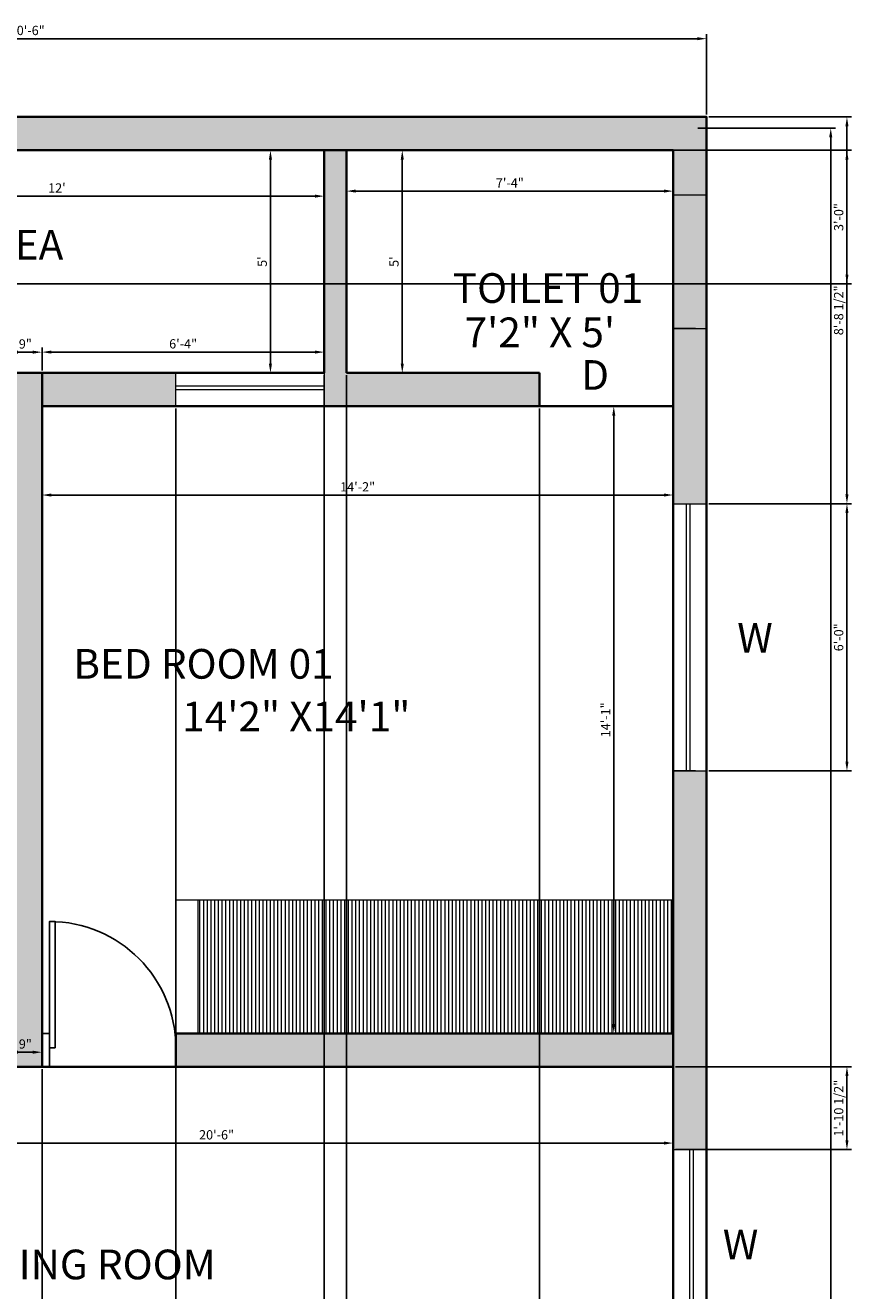
# Model space of a CAD drawing. Units: inches. Extents: x 844 to 1293, y 1224 to 2014.
# Tile 4 of 4: x 1070 to 1293, y 1673 to 2014. Entities that reach past the tile are written whole.
import ezdxf

# ---------------------------------------------------------------- set-up
doc = ezdxf.new("R2010")
doc.units = ezdxf.units.IN
for name, color, linetype, lineweight in [('A-ANNO-DIMS', 2, 'Continuous', 18), ('A-ANNO-TEXT', 3, 'Continuous', 18), ('A-AREA-IDEN', 7, 'Continuous', 25), ('A-DOOR', 3, 'Continuous', 25), ('A-FLOR-PATT', 8, 'Continuous', 13), ('A-GLAZ', 4, 'Continuous', 18), ('A-WALL', 7, 'Continuous', 35), ('A-WALL-PATT', 252, 'Continuous', 13)]:
    doc.layers.add(name, color=color, linetype=linetype, lineweight=lineweight)
doc.styles.get("Standard").update_dxf_attribs({"font": 'arial.ttf'})
doc.dimstyles.new('Copy of ISO-25', dxfattribs={"dimtxt": 2.5, "dimasz": 2.5, "dimexe": 1.25, "dimexo": 0.625, "dimtad": 1, "dimlunit": 4, "dimtxsty": 'Standard', "dimcen": 2.5, "dimadec": 0, "dimazin": 0, "dimtfac": 1, "dimtmove": 0, "dimatfit": 3, "dimfxl": 1, "dimarcsym": 0})

# ---------------------------------------------------------------- blocks, each defined once
blk = doc.blocks.new('*U3')
for p, q in [((0, 0), (0, -6)), ((40, 0), (40, -6))]:
    blk.add_line(p, q)
blk.add_lwpolyline([(0, 0), (0, 40), (1.75, 40), (1.75, 0)], close=True)
blk.add_arc((0, 0), 40, 0, 90)
blk = doc.blocks.new('*D5')
at = {"layer": 'A-ANNO-DIMS', "color": 0, "lineweight": -2, "transparency": 16777216}
for p, q in [((1074.46, 1910.42), (1074.46, 1885.88)), ((1244.46, 1910.42), (1244.46, 1885.88)), ((1076.96, 1887.13), (1241.96, 1887.13))]:
    blk.add_line(p, q, dxfattribs=at)
at = {"layer": 'A-ANNO-DIMS', "color": 0, "transparency": 16777216}
for points in [[(1076.96, 1887.54), (1076.96, 1886.71), (1074.46, 1887.13)], [(1241.96, 1887.54), (1241.96, 1886.71), (1244.46, 1887.13)]]:
    blk.add_solid(points, dxfattribs=at)
at = {"layer": 'Defpoints', "color": 0, "transparency": 16777216}
for p in [(1074.46, 1911.04), (1244.46, 1911.04), (1244.46, 1887.13)]:
    blk.add_point(p, dxfattribs=at)
at = {"layer": 'A-ANNO-DIMS', "color": 0, "transparency": 16777216, "insert": (1159.46, 1889.01), "char_height": 2.5, "attachment_point": 5}
blk.add_mtext('14\'-2"', dxfattribs=at)
blk = doc.blocks.new('*D6')
at = {"layer": 'A-ANNO-DIMS', "color": 0, "lineweight": -2, "transparency": 16777216}
for p, q in [((1243.84, 1911.04), (1227.21, 1911.04)), ((1228.46, 1908.54), (1228.46, 1744.54)), ((1243.84, 1742.04), (1227.21, 1742.04))]:
    blk.add_line(p, q, dxfattribs=at)
at = {"layer": 'A-ANNO-DIMS', "color": 0, "transparency": 16777216}
for points in [[(1228.05, 1908.54), (1228.88, 1908.54), (1228.46, 1911.04)], [(1228.05, 1744.54), (1228.88, 1744.54), (1228.46, 1742.04)]]:
    blk.add_solid(points, dxfattribs=at)
at = {"layer": 'Defpoints', "color": 0, "transparency": 16777216}
for p in [(1244.46, 1911.04), (1228.46, 1742.04), (1244.46, 1742.04)]:
    blk.add_point(p, dxfattribs=at)
at = {"layer": 'A-ANNO-DIMS', "color": 0, "transparency": 16777216, "insert": (1226.58, 1826.54), "char_height": 2.5, "attachment_point": 5, "rotation": 90}
blk.add_mtext('14\'-1"', dxfattribs=at)
blk = doc.blocks.new('*D11')
at = {"layer": 'A-ANNO-DIMS', "color": 0, "lineweight": -2, "transparency": 16777216}
for p, q in [((1006.46, 1979.42), (1006.46, 1966.44)), ((1150.46, 1979.42), (1150.46, 1966.44)), ((1008.96, 1967.69), (1147.96, 1967.69))]:
    blk.add_line(p, q, dxfattribs=at)
at = {"layer": 'A-ANNO-DIMS', "color": 0, "transparency": 16777216}
for points in [[(1008.96, 1968.11), (1008.96, 1967.27), (1006.46, 1967.69)], [(1147.96, 1968.11), (1147.96, 1967.27), (1150.46, 1967.69)]]:
    blk.add_solid(points, dxfattribs=at)
at = {"layer": 'Defpoints', "color": 0, "transparency": 16777216}
for p in [(1006.46, 1980.04), (1150.46, 1980.04), (1150.46, 1967.69)]:
    blk.add_point(p, dxfattribs=at)
at = {"layer": 'A-ANNO-DIMS', "color": 0, "transparency": 16777216, "insert": (1078.46, 1969.57), "char_height": 2.5, "attachment_point": 5}
blk.add_mtext("12'", dxfattribs=at)
blk = doc.blocks.new('*D12')
at = {"layer": 'A-ANNO-DIMS', "color": 0, "lineweight": -2, "transparency": 16777216}
for p, q in [((1149.84, 1980.04), (1134.73, 1980.04)), ((1135.98, 1922.54), (1135.98, 1977.54)), ((1149.84, 1920.04), (1134.73, 1920.04))]:
    blk.add_line(p, q, dxfattribs=at)
at = {"layer": 'A-ANNO-DIMS', "color": 0, "transparency": 16777216}
for points in [[(1135.56, 1977.54), (1136.39, 1977.54), (1135.98, 1980.04)], [(1135.56, 1922.54), (1136.39, 1922.54), (1135.98, 1920.04)]]:
    blk.add_solid(points, dxfattribs=at)
at = {"layer": 'Defpoints', "color": 0, "transparency": 16777216}
for p in [(1135.98, 1980.04), (1150.46, 1980.04), (1150.46, 1920.04)]:
    blk.add_point(p, dxfattribs=at)
at = {"layer": 'A-ANNO-DIMS', "color": 0, "transparency": 16777216, "insert": (1134.08, 1950.04), "char_height": 2.5, "attachment_point": 5, "rotation": 90}
blk.add_mtext("5'", dxfattribs=at)
blk = doc.blocks.new('*D13')
at = {"layer": 'A-ANNO-DIMS', "color": 0, "lineweight": -2, "transparency": 16777216}
for p, q in [((1156.46, 1979.42), (1156.46, 1967.79)), ((1244.46, 1979.42), (1244.46, 1967.79)), ((1158.96, 1969.04), (1241.96, 1969.04))]:
    blk.add_line(p, q, dxfattribs=at)
at = {"layer": 'A-ANNO-DIMS', "color": 0, "transparency": 16777216}
for points in [[(1158.96, 1969.46), (1158.96, 1968.63), (1156.46, 1969.04)], [(1241.96, 1969.46), (1241.96, 1968.63), (1244.46, 1969.04)]]:
    blk.add_solid(points, dxfattribs=at)
at = {"layer": 'Defpoints', "color": 0, "transparency": 16777216}
for p in [(1156.46, 1980.04), (1244.46, 1980.04), (1244.46, 1969.04)]:
    blk.add_point(p, dxfattribs=at)
at = {"layer": 'A-ANNO-DIMS', "color": 0, "transparency": 16777216, "insert": (1200.46, 1970.92), "char_height": 2.5, "attachment_point": 5}
blk.add_mtext('7\'-4"', dxfattribs=at)
blk = doc.blocks.new('*D14')
at = {"layer": 'A-ANNO-DIMS', "color": 0, "lineweight": -2, "transparency": 16777216}
for p, q in [((1157.09, 1980.04), (1172.74, 1980.04)), ((1171.49, 1977.54), (1171.49, 1922.54)), ((1157.09, 1920.04), (1172.74, 1920.04))]:
    blk.add_line(p, q, dxfattribs=at)
at = {"layer": 'A-ANNO-DIMS', "color": 0, "transparency": 16777216}
for points in [[(1171.07, 1977.54), (1171.91, 1977.54), (1171.49, 1980.04)], [(1171.07, 1922.54), (1171.91, 1922.54), (1171.49, 1920.04)]]:
    blk.add_solid(points, dxfattribs=at)
at = {"layer": 'Defpoints', "color": 0, "transparency": 16777216}
for p in [(1156.46, 1980.04), (1156.46, 1920.04), (1171.49, 1920.04)]:
    blk.add_point(p, dxfattribs=at)
at = {"layer": 'A-ANNO-DIMS', "color": 0, "transparency": 16777216, "insert": (1169.59, 1950.04), "char_height": 2.5, "attachment_point": 5, "rotation": 90}
blk.add_mtext("5'", dxfattribs=at)
blk = doc.blocks.new('*D18')
at = {"layer": 'A-ANNO-DIMS', "color": 0, "lineweight": -2, "transparency": 16777216}
for p, q in [((998.46, 1732.42), (998.46, 1711.23)), ((1244.46, 1732.42), (1244.46, 1711.23)), ((1000.96, 1712.48), (1241.96, 1712.48))]:
    blk.add_line(p, q, dxfattribs=at)
at = {"layer": 'A-ANNO-DIMS', "color": 0, "transparency": 16777216}
for points in [[(1000.96, 1712.89), (1000.96, 1712.06), (998.46, 1712.48)], [(1241.96, 1712.89), (1241.96, 1712.06), (1244.46, 1712.48)]]:
    blk.add_solid(points, dxfattribs=at)
at = {"layer": 'Defpoints', "color": 0, "transparency": 16777216}
for p in [(998.46, 1733.04), (1244.46, 1733.04), (1244.46, 1712.48)]:
    blk.add_point(p, dxfattribs=at)
at = {"layer": 'A-ANNO-DIMS', "color": 0, "transparency": 16777216, "insert": (1121.46, 1714.38), "char_height": 2.5, "attachment_point": 5}
blk.add_mtext('20\'-6"', dxfattribs=at)
blk = doc.blocks.new('*D20')
at = {"layer": 'A-ANNO-DIMS', "color": 0, "lineweight": -2, "transparency": 16777216}
for p, q in [((1251.09, 1986.04), (1288.15, 1986.04)), ((1286.9, 1983.54), (1286.9, 1268.54)), ((1251.09, 1266.04), (1288.15, 1266.04))]:
    blk.add_line(p, q, dxfattribs=at)
at = {"layer": 'A-ANNO-DIMS', "color": 0, "transparency": 16777216}
for points in [[(1286.48, 1983.54), (1287.31, 1983.54), (1286.9, 1986.04)], [(1286.48, 1268.54), (1287.31, 1268.54), (1286.9, 1266.04)]]:
    blk.add_solid(points, dxfattribs=at)
at = {"layer": 'Defpoints', "color": 0, "transparency": 16777216}
for p in [(1250.46, 1986.04), (1250.46, 1266.04), (1286.9, 1266.04)]:
    blk.add_point(p, dxfattribs=at)
at = {"layer": 'A-ANNO-DIMS', "color": 0, "transparency": 16777216, "insert": (1285, 1626.04), "char_height": 2.5, "attachment_point": 5, "rotation": 90}
blk.add_mtext("60'", dxfattribs=at)
blk = doc.blocks.new('*D27')
at = {"layer": 'A-ANNO-DIMS', "color": 0, "lineweight": -2, "transparency": 16777216}
for p, q in [((1074.46, 1920.67), (1074.46, 1926.9)), ((1150.46, 1920.67), (1150.46, 1926.9)), ((1076.96, 1925.65), (1147.96, 1925.65))]:
    blk.add_line(p, q, dxfattribs=at)
at = {"layer": 'A-ANNO-DIMS', "color": 0, "transparency": 16777216}
for points in [[(1076.96, 1926.07), (1076.96, 1925.24), (1074.46, 1925.65)], [(1147.96, 1926.07), (1147.96, 1925.24), (1150.46, 1925.65)]]:
    blk.add_solid(points, dxfattribs=at)
at = {"layer": 'Defpoints', "color": 0, "transparency": 16777216}
for p in [(1150.46, 1925.65), (1074.46, 1920.04), (1150.46, 1920.04)]:
    blk.add_point(p, dxfattribs=at)
at = {"layer": 'A-ANNO-DIMS', "color": 0, "transparency": 16777216, "insert": (1112.46, 1927.56), "char_height": 2.5, "attachment_point": 5}
blk.add_mtext('6\'-4"', dxfattribs=at)
blk = doc.blocks.new('*D30')
at = {"layer": 'A-ANNO-DIMS', "color": 0, "lineweight": -2, "transparency": 16777216}
for p, q in [((887.46, 1989.67), (887.46, 2011.37)), ((889.96, 2010.12), (1250.96, 2010.12)), ((1253.46, 1989.67), (1253.46, 2011.37))]:
    blk.add_line(p, q, dxfattribs=at)
at = {"layer": 'A-ANNO-DIMS', "color": 0, "transparency": 16777216}
for points in [[(889.96, 2010.54), (889.96, 2009.71), (887.46, 2010.12)], [(1250.96, 2010.54), (1250.96, 2009.71), (1253.46, 2010.12)]]:
    blk.add_solid(points, dxfattribs=at)
at = {"layer": 'Defpoints', "color": 0, "transparency": 16777216}
for p in [(1253.46, 2010.12), (887.46, 1989.04), (1253.46, 1989.04)]:
    blk.add_point(p, dxfattribs=at)
at = {"layer": 'A-ANNO-DIMS', "color": 0, "transparency": 16777216, "insert": (1070.46, 2012.02), "char_height": 2.5, "attachment_point": 5}
blk.add_mtext('30\'-6"', dxfattribs=at)
blk = doc.blocks.new('*D34')
at = {"layer": 'A-ANNO-DIMS', "color": 0, "lineweight": -2, "transparency": 16777216}
for p, q in [((1065.46, 1920.67), (1065.46, 1926.88)), ((1074.46, 1920.67), (1074.46, 1926.88)), ((1067.96, 1925.63), (1071.96, 1925.63))]:
    blk.add_line(p, q, dxfattribs=at)
at = {"layer": 'A-ANNO-DIMS', "color": 0, "transparency": 16777216}
for points in [[(1067.96, 1926.05), (1067.96, 1925.22), (1065.46, 1925.63)], [(1071.96, 1926.05), (1071.96, 1925.22), (1074.46, 1925.63)]]:
    blk.add_solid(points, dxfattribs=at)
at = {"layer": 'Defpoints', "color": 0, "transparency": 16777216}
for p in [(1074.46, 1925.63), (1065.46, 1920.04), (1074.46, 1920.04)]:
    blk.add_point(p, dxfattribs=at)
at = {"layer": 'A-ANNO-DIMS', "color": 0, "transparency": 16777216, "insert": (1069.96, 1927.53), "char_height": 2.5, "attachment_point": 5}
blk.add_mtext('9"', dxfattribs=at)
blk = doc.blocks.new('*D36')
at = {"layer": 'A-ANNO-DIMS', "color": 0, "lineweight": -2, "transparency": 16777216}
for p, q in [((1065.46, 1733.67), (1065.46, 1738.21)), ((1067.96, 1736.96), (1071.96, 1736.96)), ((1074.46, 1733.67), (1074.46, 1738.21))]:
    blk.add_line(p, q, dxfattribs=at)
at = {"layer": 'A-ANNO-DIMS', "color": 0, "transparency": 16777216}
for points in [[(1067.96, 1737.38), (1067.96, 1736.54), (1065.46, 1736.96)], [(1071.96, 1737.38), (1071.96, 1736.54), (1074.46, 1736.96)]]:
    blk.add_solid(points, dxfattribs=at)
at = {"layer": 'Defpoints', "color": 0, "transparency": 16777216}
for p in [(1074.46, 1736.96), (1065.46, 1733.04), (1074.46, 1733.04)]:
    blk.add_point(p, dxfattribs=at)
at = {"layer": 'A-ANNO-DIMS', "color": 0, "transparency": 16777216, "insert": (1069.96, 1738.86), "char_height": 2.5, "attachment_point": 5}
blk.add_mtext('9"', dxfattribs=at)
blk = doc.blocks.new('WIN-GLAZ-60IN')
for p, q in [((0, 60), (0, 0)), ((1, 60), (1, 0))]:
    blk.add_line(p, q)
blk = doc.blocks.new('*D55')
at = {"layer": 'A-ANNO-DIMS', "color": 0, "lineweight": -2, "transparency": 16777216}
for p, q in [((1254.09, 1989.04), (1292.51, 1989.04)), ((1291.26, 1887.28), (1291.26, 1986.54)), ((1254.09, 1884.78), (1292.51, 1884.78))]:
    blk.add_line(p, q, dxfattribs=at)
at = {"layer": 'A-ANNO-DIMS', "color": 0, "transparency": 16777216}
for points in [[(1290.85, 1986.54), (1291.68, 1986.54), (1291.26, 1989.04)], [(1290.85, 1887.28), (1291.68, 1887.28), (1291.26, 1884.78)]]:
    blk.add_solid(points, dxfattribs=at)
at = {"layer": 'Defpoints', "color": 0, "transparency": 16777216}
for p in [(1253.46, 1989.04), (1291.26, 1989.04), (1253.46, 1884.78)]:
    blk.add_point(p, dxfattribs=at)
at = {"layer": 'A-ANNO-DIMS', "color": 0, "transparency": 16777216, "insert": (1289.35, 1936.91), "char_height": 2.5, "attachment_point": 5, "rotation": 90}
blk.add_mtext('8\'-8 1/2"', dxfattribs=at)
blk = doc.blocks.new('*D56')
at = {"layer": 'A-ANNO-DIMS', "color": 0, "lineweight": -2, "transparency": 16777216}
for p, q in [((1254.09, 1884.78), (1292.51, 1884.78)), ((1291.26, 1815.28), (1291.26, 1882.28)), ((1254.09, 1812.78), (1292.51, 1812.78))]:
    blk.add_line(p, q, dxfattribs=at)
at = {"layer": 'A-ANNO-DIMS', "color": 0, "transparency": 16777216}
for points in [[(1290.85, 1882.28), (1291.68, 1882.28), (1291.26, 1884.78)], [(1290.85, 1815.28), (1291.68, 1815.28), (1291.26, 1812.78)]]:
    blk.add_solid(points, dxfattribs=at)
at = {"layer": 'Defpoints', "color": 0, "transparency": 16777216}
for p in [(1253.46, 1884.78), (1291.26, 1884.78), (1253.46, 1812.78)]:
    blk.add_point(p, dxfattribs=at)
at = {"layer": 'A-ANNO-DIMS', "color": 0, "transparency": 16777216, "insert": (1289.36, 1848.78), "char_height": 2.5, "attachment_point": 5, "rotation": 90}
blk.add_mtext('6\'-0"', dxfattribs=at)
blk = doc.blocks.new('*D58')
at = {"layer": 'A-ANNO-DIMS', "color": 0, "lineweight": -2, "transparency": 16777216}
for p, q in [((1245.09, 1733.04), (1292.51, 1733.04)), ((1291.26, 1713.23), (1291.26, 1730.54)), ((1245.09, 1710.73), (1292.51, 1710.73))]:
    blk.add_line(p, q, dxfattribs=at)
at = {"layer": 'A-ANNO-DIMS', "color": 0, "transparency": 16777216}
for points in [[(1290.85, 1730.54), (1291.68, 1730.54), (1291.26, 1733.04)], [(1290.85, 1713.23), (1291.68, 1713.23), (1291.26, 1710.73)]]:
    blk.add_solid(points, dxfattribs=at)
at = {"layer": 'Defpoints', "color": 0, "transparency": 16777216}
for p in [(1244.46, 1733.04), (1291.26, 1733.04), (1244.46, 1710.73)]:
    blk.add_point(p, dxfattribs=at)
at = {"layer": 'A-ANNO-DIMS', "color": 0, "transparency": 16777216, "insert": (1289.35, 1721.88), "char_height": 2.5, "attachment_point": 5, "rotation": 90}
blk.add_mtext('1\'-10 1/2"', dxfattribs=at)
blk = doc.blocks.new('*D63')
at = {"layer": 'A-ANNO-DIMS', "color": 0, "lineweight": -2, "transparency": 16777216}
for p, q in [((1110.46, 1910.42), (1110.46, 1223.99)), ((1150.46, 1910.42), (1150.46, 1223.99)), ((1112.96, 1225.24), (1147.96, 1225.24))]:
    blk.add_line(p, q, dxfattribs=at)
at = {"layer": 'A-ANNO-DIMS', "color": 0, "transparency": 16777216}
for points in [[(1112.96, 1225.66), (1112.96, 1224.82), (1110.46, 1225.24)], [(1147.96, 1225.66), (1147.96, 1224.82), (1150.46, 1225.24)]]:
    blk.add_solid(points, dxfattribs=at)
at = {"layer": 'Defpoints', "color": 0, "transparency": 16777216}
for p in [(1110.46, 1911.04), (1150.46, 1911.04), (1150.46, 1225.24)]:
    blk.add_point(p, dxfattribs=at)
at = {"layer": 'A-ANNO-DIMS', "color": 0, "transparency": 16777216, "insert": (1130.46, 1227.14), "char_height": 2.5, "attachment_point": 5}
blk.add_mtext('3\'-4"', dxfattribs=at)
blk = doc.blocks.new('*D64')
at = {"layer": 'A-ANNO-DIMS', "color": 0, "lineweight": -2, "transparency": 16777216}
for p, q in [((1208.46, 1910.42), (1208.46, 1223.99)), ((1244.46, 1910.42), (1244.46, 1223.99)), ((1210.96, 1225.24), (1241.96, 1225.24))]:
    blk.add_line(p, q, dxfattribs=at)
at = {"layer": 'A-ANNO-DIMS', "color": 0, "transparency": 16777216}
for points in [[(1210.96, 1225.66), (1210.96, 1224.82), (1208.46, 1225.24)], [(1241.96, 1225.66), (1241.96, 1224.82), (1244.46, 1225.24)]]:
    blk.add_solid(points, dxfattribs=at)
at = {"layer": 'Defpoints', "color": 0, "transparency": 16777216}
for p in [(1208.46, 1911.04), (1244.46, 1911.04), (1244.46, 1225.24)]:
    blk.add_point(p, dxfattribs=at)
at = {"layer": 'A-ANNO-DIMS', "color": 0, "transparency": 16777216, "insert": (1226.46, 1227.14), "char_height": 2.5, "attachment_point": 5}
blk.add_mtext('3\'-0"', dxfattribs=at)
blk = doc.blocks.new('*D65')
at = {"layer": 'A-ANNO-DIMS', "color": 0, "lineweight": -2, "transparency": 16777216}
for p, q in [((1007.09, 1980.04), (1292.51, 1980.04)), ((1291.26, 1946.54), (1291.26, 1977.54)), ((1001.09, 1944.04), (1292.51, 1944.04))]:
    blk.add_line(p, q, dxfattribs=at)
at = {"layer": 'A-ANNO-DIMS', "color": 0, "transparency": 16777216}
for points in [[(1290.85, 1977.54), (1291.68, 1977.54), (1291.26, 1980.04)], [(1290.85, 1946.54), (1291.68, 1946.54), (1291.26, 1944.04)]]:
    blk.add_solid(points, dxfattribs=at)
at = {"layer": 'Defpoints', "color": 0, "transparency": 16777216}
for p in [(1006.46, 1980.04), (1291.26, 1980.04), (1000.46, 1944.04)]:
    blk.add_point(p, dxfattribs=at)
at = {"layer": 'A-ANNO-DIMS', "color": 0, "transparency": 16777216, "insert": (1289.36, 1962.04), "char_height": 2.5, "attachment_point": 5, "rotation": 90}
blk.add_mtext('3\'-0"', dxfattribs=at)
blk = doc.blocks.new('*D67')
at = {"layer": 'A-ANNO-DIMS', "color": 0, "lineweight": -2, "transparency": 16777216}
for p, q in [((1074.46, 1732.42), (1074.46, 1223.99)), ((1110.46, 1732.42), (1110.46, 1223.99)), ((1076.96, 1225.24), (1107.96, 1225.24))]:
    blk.add_line(p, q, dxfattribs=at)
at = {"layer": 'A-ANNO-DIMS', "color": 0, "transparency": 16777216}
for points in [[(1076.96, 1225.66), (1076.96, 1224.82), (1074.46, 1225.24)], [(1107.96, 1225.66), (1107.96, 1224.82), (1110.46, 1225.24)]]:
    blk.add_solid(points, dxfattribs=at)
at = {"layer": 'Defpoints', "color": 0, "transparency": 16777216}
for p in [(1074.46, 1733.04), (1110.46, 1733.04), (1110.46, 1225.24)]:
    blk.add_point(p, dxfattribs=at)
at = {"layer": 'A-ANNO-DIMS', "color": 0, "transparency": 16777216, "insert": (1092.46, 1227.14), "char_height": 2.5, "attachment_point": 5}
blk.add_mtext('3\'-0"', dxfattribs=at)
blk = doc.blocks.new('*D73')
at = {"layer": 'A-ANNO-DIMS', "color": 0, "lineweight": -2, "transparency": 16777216}
for p, q in [((1150.46, 1919.42), (1150.46, 1223.99)), ((1156.46, 1919.42), (1156.46, 1223.99)), ((1147.96, 1225.24), (1145.46, 1225.24)), ((1150.46, 1225.24), (1156.46, 1225.24)), ((1158.96, 1225.24), (1169.36, 1225.24))]:
    blk.add_line(p, q, dxfattribs=at)
at = {"layer": 'A-ANNO-DIMS', "color": 0, "transparency": 16777216}
for points in [[(1147.96, 1225.66), (1147.96, 1224.82), (1150.46, 1225.24)], [(1158.96, 1225.66), (1158.96, 1224.82), (1156.46, 1225.24)]]:
    blk.add_solid(points, dxfattribs=at)
at = {"layer": 'Defpoints', "color": 0, "transparency": 16777216}
for p in [(1150.46, 1920.04), (1156.46, 1920.04), (1156.46, 1225.24)]:
    blk.add_point(p, dxfattribs=at)
at = {"layer": 'A-ANNO-DIMS', "color": 0, "transparency": 16777216, "insert": (1165.41, 1227.14), "char_height": 2.5, "attachment_point": 5}
blk.add_mtext('0\'-6"', dxfattribs=at)

msp = doc.modelspace()

# ---------------------------------------------------------------- hatches: boundary and pattern name
at = {"layer": 'A-FLOR-PATT'}
h = msp.add_hatch(dxfattribs=at)
h.set_pattern_fill('ANSI31', color=256, scale=0.3149606, angle=45, style=0)
h.paths.add_polyline_path([(1116.465, 1742.042), (1244.465, 1742.042), (1244.465, 1778.042), (1116.465, 1778.042)])
at = {"layer": 'A-WALL-PATT'}
h = msp.add_hatch(color=256, dxfattribs=at)
h.dxf.hatch_style = 1
h.paths.add_polyline_path([(1253.465, 1989.042), (887.465, 1989.042), (887.465, 1920.042), (887.465, 1911.042), (887.465, 1871.621), (896.465, 1871.621), (896.465, 1911.042), (896.465, 1920.042), (896.465, 1980.042), (1000.465, 1980.042), (1244.465, 1980.042), (1244.465, 1968.042), (1253.465, 1968.042)])
h.paths.add_polyline_path([(1006.465, 1944.042), (1000.465, 1944.042), (1000.465, 1920.042), (896.465, 1920.042), (896.465, 1911.042), (1006.465, 1911.042), (1006.465, 1920.042)], flags=17)
h.paths.add_polyline_path([(1253.465, 1968.042), (1244.465, 1968.042), (1244.465, 1932.042), (1253.465, 1932.042)], flags=17)
h.paths.add_polyline_path([(1253.465, 1920.042), (1253.465, 1932.042), (1244.465, 1932.042), (1244.465, 1920.042), (1244.465, 1911.042), (1244.465, 1884.775), (1253.465, 1884.775), (1253.465, 1911.042)], flags=17)
h.paths.add_polyline_path([(1208.465, 1920.042), (1156.465, 1920.042), (1156.465, 1980.042), (1150.465, 1980.042), (1150.465, 1920.042), (1150.465, 1911.042), (1208.465, 1911.042)], flags=17)
h.paths.add_polyline_path([(1110.465, 1920.042), (1074.465, 1920.042), (1074.465, 1911.042), (1110.465, 1911.042)], flags=17)
h.paths.add_polyline_path([(896.465, 1811.621), (887.465, 1811.621), (887.465, 1672.343), (896.465, 1672.343), (896.465, 1733.042), (896.465, 1742.042)])
h.paths.add_polyline_path([(896.465, 1624.343), (887.465, 1624.343), (887.465, 1263.042), (1253.465, 1263.042), (1253.465, 1574.212), (1244.465, 1574.212), (1244.465, 1563.042), (1244.465, 1554.042), (1244.465, 1272.042), (1016.465, 1272.042), (1016.465, 1267.542), (896.465, 1267.542), (896.465, 1272.042), (896.465, 1554.042), (968.465, 1554.042), (989.465, 1554.042), (998.465, 1554.042), (998.465, 1623.042), (989.465, 1623.042), (989.465, 1563.042), (896.465, 1563.042)])
h.paths.add_polyline_path([(998.465, 1518.042), (994.855, 1518.042), (989.465, 1518.042), (989.465, 1497.104), (998.465, 1497.104)], flags=17)
h.paths.add_polyline_path([(998.465, 1449.104), (989.465, 1449.104), (989.465, 1391.042), (998.465, 1391.042), (1070.313, 1391.042), (1070.313, 1396.464), (1070.313, 1400.042), (998.465, 1400.042)], flags=17)
h.paths.add_polyline_path([(1112.465, 1450.531), (1106.465, 1450.531), (1106.465, 1400.042), (1106.465, 1391.042), (1112.465, 1391.042)], flags=17)
h.paths.add_polyline_path([(1112.465, 1554.042), (1112.394, 1554.042), (1112.394, 1559.602, -0.015479), (1112.465, 1561.896), (1112.465, 1563.042), (1106.465, 1563.042), (1106.465, 1554.042), (1106.465, 1510.531), (1112.465, 1510.531)], flags=17)
h.paths.add_polyline_path([(1158.465, 1623.042), (1244.465, 1623.042), (1244.465, 1632.042), (1158.465, 1632.042), (1149.465, 1632.042), (1149.465, 1599.042), (1158.465, 1599.042)])
h.paths.add_polyline_path([(1244.465, 1563.042), (1158.465, 1563.042), (1149.465, 1563.042), (1149.465, 1554.042), (1244.465, 1554.042)], flags=17)
h.paths.add_polyline_path([(1253.465, 1650.728), (1244.465, 1650.728), (1244.465, 1610.212), (1253.465, 1610.212)])
h.paths.add_polyline_path([(998.465, 1733.042), (989.465, 1733.042), (989.465, 1673.042), (998.465, 1673.042)])
h.paths.add_polyline_path([(1029.465, 1742.042), (896.465, 1742.042), (896.465, 1733.042), (989.465, 1733.042), (1029.465, 1733.042)])
h.paths.add_polyline_path([(1244.465, 1742.042), (1110.465, 1742.042), (1110.465, 1739.692, -0.0113533), (1110.5, 1738.147), (1110.5, 1733.042), (1244.465, 1733.042)])
h.paths.add_polyline_path([(1253.465, 1812.775), (1244.465, 1812.775), (1244.465, 1710.728), (1253.465, 1710.728)])
h.paths.add_polyline_path([(1074.465, 1911.042), (1074.465, 1920.042), (1065.465, 1920.042), (1065.465, 1911.042), (1065.465, 1742.042), (1065.465, 1733.042), (1074.465, 1733.042), (1074.465, 1742.042)])
h.paths.add_polyline_path([(1067.758, 1736.261), (1072.19, 1736.261), (1072.19, 1741.413), (1067.758, 1741.413)], flags=24)
h.paths.add_polyline_path([(975.783, 1886.472), (985.93, 1886.472), (985.93, 1891.624), (975.783, 1891.624)], flags=25)
h.paths.add_polyline_path([(917.205, 1821.36), (917.205, 1831.507), (912.053, 1831.507), (912.053, 1821.36)], flags=9)
h.paths.add_polyline_path([(1050.545, 1543.381), (1054.404, 1543.381), (1054.404, 1548.533), (1050.545, 1548.533)], flags=25)
h.paths.add_polyline_path([(1116.422, 1711.778), (1126.569, 1711.778), (1126.569, 1716.93), (1116.422, 1716.93)], flags=9)
h.paths.add_polyline_path([(1019.298, 1637.389), (1019.298, 1649.478), (1014.146, 1649.478), (1014.146, 1637.389)], flags=9)
h.paths.add_polyline_path([(980.864, 1534.121), (980.864, 1537.98), (975.712, 1537.98), (975.712, 1534.121)], flags=25)
h.paths.add_polyline_path([(1019.234, 1470.889), (1019.234, 1482.978), (1014.082, 1482.978), (1014.082, 1470.889)], flags=25)
h.paths.add_polyline_path([(1175.456, 1538.714), (1181.257, 1538.714), (1181.257, 1543.865), (1175.456, 1543.865)], flags=25)
h.paths.add_polyline_path([(1122.736, 1467.36), (1122.736, 1477.507), (1117.584, 1477.507), (1117.584, 1467.36)], flags=25)
h.paths.add_polyline_path([(907.276, 1556.335), (907.276, 1560.767), (902.124, 1560.767), (902.124, 1556.335)], flags=24)
h.paths.add_polyline_path([(1107.309, 1567.013), (1111.742, 1567.013), (1111.742, 1572.165), (1107.309, 1572.165)], flags=25)
h.paths.add_polyline_path([(955.783, 1784.038), (965.93, 1784.038), (965.93, 1789.19), (955.783, 1789.19)], flags=9)
h.paths.add_polyline_path([(1004.344, 1643.999), (1004.344, 1652.203), (999.192, 1652.203), (999.192, 1643.999)], flags=9)
h.paths.add_polyline_path([(973.263, 1534.121), (973.263, 1537.98), (968.111, 1537.98), (968.111, 1534.121)], flags=25)
h.paths.add_polyline_path([(1047.536, 1660.728), (1114.78, 1660.728), (1114.78, 1672.982), (1047.536, 1672.982)], flags=9)
h.paths.add_polyline_path([(1047.509, 1673.552), (1128.636, 1673.552), (1128.636, 1685.969), (1047.509, 1685.969)], flags=9)
h.paths.add_polyline_path([(999.825, 1474.75), (1014.374, 1474.75), (1014.374, 1486.75), (999.825, 1486.75)], flags=25)
h.paths.add_polyline_path([(1085.974, 1473.689), (1100.523, 1473.689), (1100.523, 1485.689), (1085.974, 1485.689)], flags=25)
h.paths.add_polyline_path([(898.914, 1844.786), (913.462, 1844.786), (913.462, 1856.786), (898.914, 1856.786)], flags=9)
h.paths.add_polyline_path([(1021.801, 1899.15), (1036.35, 1899.15), (1036.35, 1911.15), (1021.801, 1911.15)], flags=25)
h.paths.add_polyline_path([(933.371, 1817.465), (997.445, 1817.465), (997.445, 1829.522), (933.371, 1829.522)], flags=9)
h.paths.add_polyline_path([(912.536, 1375.627), (960.277, 1375.627), (960.277, 1387.881), (912.536, 1387.881)], flags=25)
h.paths.add_polyline_path([(908.723, 1393.944), (979.923, 1393.944), (979.923, 1406.361), (908.723, 1406.361)], flags=25)
h.paths.add_polyline_path([(907.199, 1415.111), (926.792, 1415.111), (926.792, 1427.316), (907.199, 1427.316)], flags=25)
h.paths.add_polyline_path([(1130.034, 1467.266), (1180.017, 1467.266), (1180.017, 1479.52), (1130.034, 1479.52)], flags=25)
h.paths.add_polyline_path([(1130.007, 1480.09), (1210.517, 1480.09), (1210.517, 1492.508), (1130.007, 1492.508)], flags=25)
h.paths.add_polyline_path([(918.552, 1280.947), (1012.38, 1280.947), (1012.38, 1293.356), (918.552, 1293.356)], flags=25)
h.paths.add_polyline_path([(1074.912, 1322.783), (1119.613, 1322.783), (1119.613, 1334.988), (1074.912, 1334.988)], flags=25)
h.paths.add_polyline_path([(994.568, 1321.709), (1075.078, 1321.709), (1075.078, 1334.127), (994.568, 1334.127)], flags=25)
h.paths.add_polyline_path([(932.502, 1835.432), (1188.778, 1835.432), (1188.778, 1847.849), (932.502, 1847.849)], flags=9)

# ---------------------------------------------------------------- linework, layer by layer
at = {"layer": 'A-DOOR'}
for p, q in [((1076.465, 1742.042), (1074.465, 1742.042)), ((1076.465, 1733.042), (1076.465, 1742.042)), ((1074.465, 1733.042), (1076.465, 1733.042))]:
    msp.add_line(p, q, dxfattribs=at)
at = {"layer": 'A-FLOR-PATT'}
for p, q in [((1110.465, 1742.042), (1110.465, 1778.042)), ((1110.465, 1778.042), (1116.465, 1778.042)), ((1116.465, 1778.042), (1116.465, 1742.042)), ((1116.465, 1778.042), (1244.465, 1778.042))]:
    msp.add_line(p, q, dxfattribs=at)
at = {"layer": 'A-GLAZ'}
for p, q in [((1244.465, 1968.042), (1250.465, 1968.042)), ((1244.465, 1968.042), (1253.465, 1968.042)), ((1250.465, 1932.042), (1244.465, 1932.042)), ((1244.465, 1932.042), (1253.465, 1932.042)), ((1110.465, 1911.042), (1110.465, 1920.042)), ((1150.465, 1920.042), (1150.465, 1911.042)), ((1110.465, 1916.542), (1150.465, 1916.542)), ((1110.465, 1915.542), (1150.465, 1915.542)), ((1244.465, 1884.775), (1250.465, 1884.775)), ((1244.465, 1884.775), (1253.465, 1884.775)), ((1247.965, 1884.775), (1247.965, 1812.775)), ((1248.965, 1884.775), (1248.965, 1812.775)), ((1250.465, 1812.775), (1244.465, 1812.775)), ((1244.465, 1812.775), (1253.465, 1812.775)), ((1244.465, 1710.728), (1246.465, 1710.728)), ((1244.465, 1710.728), (1253.465, 1710.728))]:
    msp.add_line(p, q, dxfattribs=at)
at = {"layer": 'A-WALL'}
for p, q in [((1144.465, 1980.042), (1150.465, 1980.042)), ((1150.465, 1980.042), (1150.465, 1920.042)), ((1156.465, 1920.042), (1156.465, 1980.042)), ((1244.465, 1980.042), (1244.465, 1968.042)), ((1006.465, 1920.042), (1144.465, 1920.042)), ((1006.465, 1920.042), (1074.465, 1920.042)), ((1074.465, 1920.042), (1074.465, 1911.042)), ((1110.465, 1920.042), (1150.465, 1920.042)), ((1144.465, 1920.042), (1150.465, 1920.042)), ((1156.465, 1920.042), (1208.465, 1920.042)), ((1208.465, 1911.042), (1208.465, 1920.042)), ((1244.465, 1920.042), (1244.465, 1911.042)), ((1253.465, 1920.042), (1253.465, 1911.042)), ((1074.465, 1742.042), (1074.465, 1911.042)), ((1074.465, 1911.042), (1110.465, 1911.042)), ((1074.465, 1911.042), (1144.465, 1911.042)), ((1150.465, 1911.042), (1102.465, 1911.042)), ((1150.465, 1911.042), (1144.465, 1911.042)), ((1150.465, 1911.042), (1244.465, 1911.042)), ((1244.465, 1911.042), (1244.465, 1884.775)), ((1074.465, 1742.042), (1074.465, 1733.042)), ((1244.465, 1742.042), (1110.465, 1742.042)), ((1110.465, 1733.042), (1110.465, 1742.042)), ((1244.465, 1733.042), (1244.465, 1742.042)), ((1029.595, 1733.042), (1244.465, 1733.042)), ((1244.465, 1733.042), (1244.465, 1563.042)), ((1244.465, 1733.042), (1244.465, 1710.728))]:
    msp.add_line(p, q, dxfattribs=at)
for points in [[(1253.465, 1920.042), (1253.465, 1989.042), (887.465, 1989.042), (887.465, 1920.042)], [(1244.465, 1920.042), (1244.465, 1980.042), (896.465, 1980.042), (896.465, 1920.042)], [(887.465, 1911.042), (887.465, 1263.042), (1253.465, 1263.042), (1253.465, 1911.042)], [(1016.465, 1272.042), (1244.465, 1272.042), (1244.465, 1911.042)]]:
    msp.add_lwpolyline(points, dxfattribs=at)

# ---------------------------------------------------------------- block references
at = {"layer": 'A-DOOR', "xscale": 0.8508771855932021, "yscale": 0.8508771855932021, "zscale": 0.8508771855932021}
msp.add_blockref('*U3', (1076.465, 1738.147), dxfattribs=at)
at = {"layer": 'A-GLAZ', "rotation": 180}
msp.add_blockref('WIN-GLAZ-60IN', (1249.965, 1710.728), dxfattribs=at)

# ---------------------------------------------------------------- texts
at = {"layer": 'A-ANNO-TEXT'}
for s, p in [('D', (1219.675, 1915.486)), ('W', (1261.705, 1844.663)), ('W', (1257.821, 1681.177))]:
    msp.add_text(s, height=8, dxfattribs=at).set_placement(p)
at = {"layer": 'A-AREA-IDEN'}
for s, p in [('BACK AREA', (1023.293, 1950.587)), ('TOILET 01', (1185.101, 1938.913)), ('7\'2" X 5\'', (1188.272, 1926.979)), ('BED ROOM 02                                BED ROOM 01', (934.572, 1837.638)), ('14\'2" X14\'1"', (1112.222, 1823.451)), ('DINING ROOM', (1049.578, 1675.758))]:
    msp.add_text(s, height=8, dxfattribs=at).set_placement(p)

# ---------------------------------------------------------------- dimensions: what is measured, and where the dimension line sits
at = {"layer": 'A-ANNO-DIMS'}
for base, p1, p2, override, picture, middle in [((1253.465, 2010.122), (887.465, 1989.042), (1253.465, 1989.042), {"dimclrd": 0, "dimclre": 0, "dimclrt": 0}, '*D30', (1070.465, 2012.024)), ((1150.465, 1967.69), (1006.465, 1980.042), (1150.465, 1980.042), {"dimclrd": 0, "dimclre": 0, "dimclrt": 0}, '*D11', (1078.465, 1969.57)), ((1244.465, 1969.043), (1156.465, 1980.042), (1244.465, 1980.042), {"dimclrd": 0, "dimclre": 0, "dimclrt": 0}, '*D13', (1200.465, 1970.918)), ((1074.465, 1925.633), (1065.465, 1920.042), (1074.465, 1920.042), {"dimclrd": 0, "dimclre": 0, "dimclrt": 0}, '*D34', (1069.965, 1927.534)), ((1150.465, 1925.654), (1074.465, 1920.042), (1150.465, 1920.042), {"dimclrd": 0, "dimclre": 0, "dimclrt": 0}, '*D27', (1112.465, 1927.556)), ((1156.465, 1225.242), (1150.465, 1920.042), (1156.465, 1920.042), {"dimdec": 1, "dimlfac": 1, "dimrnd": 0, "dimzin": 1, "dimdsep": 46, "dimlunit": 4, "dimfrac": 2}, '*D73', (1165.413, 1227.143)), ((1244.465, 1887.128), (1074.465, 1911.042), (1244.465, 1911.042), {"dimclrd": 0, "dimclre": 0, "dimclrt": 0}, '*D5', (1159.465, 1889.008)), ((1150.465, 1225.242), (1110.465, 1911.042), (1150.465, 1911.042), {"dimdec": 1, "dimlfac": 1, "dimrnd": 0, "dimzin": 1, "dimdsep": 46, "dimlunit": 4, "dimfrac": 2}, '*D63', (1130.465, 1227.144)), ((1244.465, 1225.242), (1208.465, 1911.042), (1244.465, 1911.042), {"dimdec": 1, "dimlfac": 1, "dimrnd": 0, "dimzin": 1, "dimdsep": 46, "dimlunit": 4, "dimfrac": 2}, '*D64', (1226.465, 1227.144)), ((1074.465, 1736.959), (1065.465, 1733.042), (1074.465, 1733.042), {"dimclrd": 0, "dimclre": 0, "dimclrt": 0}, '*D36', (1069.965, 1738.86)), ((1244.465, 1712.476), (998.465, 1733.042), (1244.465, 1733.042), {"dimclrd": 0, "dimclre": 0, "dimclrt": 0}, '*D18', (1121.465, 1714.377)), ((1110.465, 1225.242), (1074.465, 1733.042), (1110.465, 1733.042), {"dimdec": 1, "dimlfac": 1, "dimrnd": 0, "dimzin": 1, "dimdsep": 46, "dimlunit": 4, "dimfrac": 2}, '*D67', (1092.465, 1227.144))]:
    dim = msp.add_linear_dim(base=base, p1=p1, p2=p2, dimstyle='Copy of ISO-25', override=override, dxfattribs=at)
    dim.commit()
    dim.dimension.update_dxf_attribs({"geometry": picture, "text_midpoint": middle})
for base, p1, p2, override, picture, middle in [((1291.265, 1989.042), (1253.465, 1884.775), (1253.465, 1989.042), {"dimdec": 1, "dimlfac": 1, "dimrnd": 0, "dimzin": 1, "dimdsep": 46, "dimlunit": 4, "dimfrac": 2}, '*D55', (1289.347, 1936.908)), ((1286.898, 1266.042), (1250.465, 1986.042), (1250.465, 1266.042), {"dimclrd": 0, "dimclre": 0, "dimclrt": 0}, '*D20', (1284.997, 1626.042)), ((1291.265, 1980.042), (1000.465, 1944.042), (1006.465, 1980.042), {"dimdec": 1, "dimlfac": 1, "dimrnd": 0, "dimzin": 1, "dimdsep": 46, "dimlunit": 4, "dimfrac": 2}, '*D65', (1289.363, 1962.042)), ((1135.978, 1980.042), (1150.465, 1920.042), (1150.465, 1980.042), {"dimclrd": 0, "dimclre": 0, "dimclrt": 0}, '*D12', (1134.081, 1950.042)), ((1171.489, 1920.042), (1156.465, 1980.042), (1156.465, 1920.042), {"dimclrd": 0, "dimclre": 0, "dimclrt": 0}, '*D14', (1169.593, 1950.042)), ((1228.465, 1742.042), (1244.465, 1911.042), (1244.465, 1742.042), {"dimclrd": 0, "dimclre": 0, "dimclrt": 0}, '*D6', (1226.585, 1826.542)), ((1291.265, 1884.775), (1253.465, 1812.775), (1253.465, 1884.775), {"dimdec": 1, "dimlfac": 1, "dimrnd": 0, "dimzin": 1, "dimdsep": 46, "dimlunit": 4, "dimfrac": 2}, '*D56', (1289.363, 1848.775)), ((1291.265, 1733.042), (1244.465, 1710.728), (1244.465, 1733.042), {"dimdec": 1, "dimlfac": 1, "dimrnd": 0, "dimzin": 1, "dimdsep": 46, "dimlunit": 4, "dimfrac": 2}, '*D58', (1289.347, 1721.885))]:
    dim = msp.add_linear_dim(base=base, p1=p1, p2=p2, angle=90, dimstyle='Copy of ISO-25', override=override, dxfattribs=at)
    dim.commit()
    dim.dimension.update_dxf_attribs({"geometry": picture, "text_midpoint": middle})

doc.saveas('drawing.dxf')
